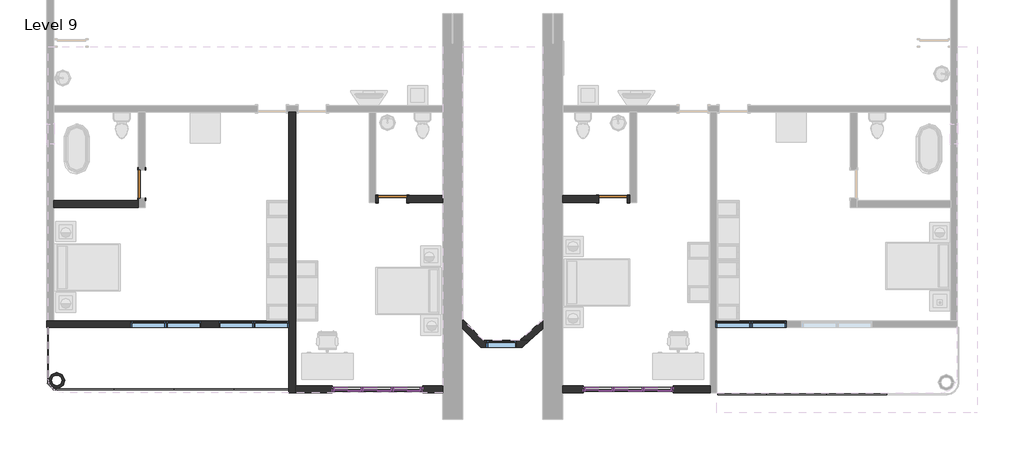
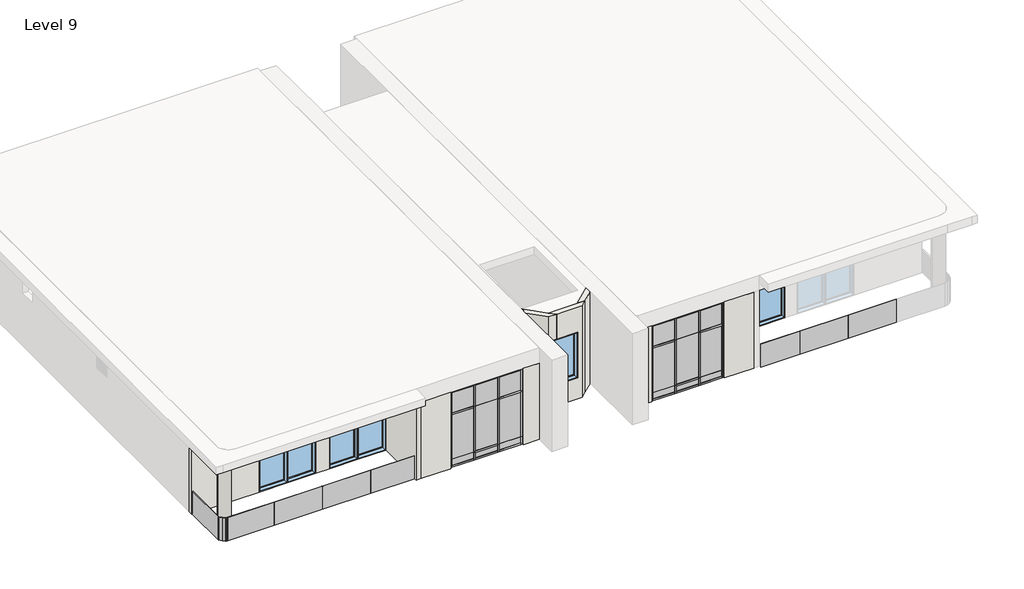
# One storey, part 1 of 3: 42 members, 30 plates, 14 walls, 7 windows, 3 doors.
"""IFC4 building model written with IfcOpenShell, lengths in millimetres."""

from ifc_helpers import new_model, si_unit, point, frame, frame_2d, origin, place, context, project, spatial, polyline, circle_curve, trimmed, segment, composite_curve, outline, extrude, faceted_brep, transform, mapped, element, save
from components import door_2703ae13, door_10fd3a06, member_c17f1be2, member_ad567e07, member_d2e7e466, member_7db1855a, member_75d1e245, member_d60e8053, member_3c3dc66a, member_2fae0574, member_410c6227, member_73c23c35, system_panel_glazed_38d54ecf, system_panel_glazed_fbb6c980, system_panel_glazed_4137532c, system_panel_glazed_6230de04, system_panel_glazed_a79f7f85, system_panel_glazed_9a5ea490, system_panel_glazed_95be5de7, system_panel_glazed_1e00a1c5, system_panel_glazed_ffe51582, system_panel_glazed_8f95e3f6, system_panel_glazed_836907cd, system_panel_glazed_688a65a2, system_panel_glazed_c1a1c740, system_panel_glazed_22bcd51f, window_9a779fa2, window_1a213a25

model = new_model("IFC4")

# Units and contexts
model_context = context("Model", 3, world=origin())
ifc_project = project(units=[si_unit("LENGTHUNIT", "METRE", prefix="MILLI")], contexts=[model_context])

# Site, building, storey
site = spatial("IfcSite", under=ifc_project)
building = spatial("IfcBuilding", under=site)
storey = spatial("IfcBuildingStorey", under=building, Name="Level 9", Elevation=29260.8)

# Doors
placement = place(None, origin())
door_shape = door_2703ae13(model_context)
element("IfcDoor", 1, ObjectType="Door-Single-Panel.0001 : 34\" x 80\"", at=placement, inside=storey, context=model_context, shape_type="MappedRepresentation", body=[
    mapped(door_shape, transform((-15765.9987704, -441.9241442, 29260.8), x_axis=(0.0, -1.0, 0.0), y_axis=(1.0, 0.0, 0.0), z_axis=(0.0, 0.0, 1.0))),
])
element("IfcDoor", 2, ObjectType="Door-Single-Panel.0001 : 34\" x 80\"", at=placement, inside=storey, context=model_context, shape_type="MappedRepresentation", body=[
    mapped(door_shape, transform((-8145.9987704, -899.1241442, 29260.8), x_axis=(-1.0, 0.0, 0.0), y_axis=(0.0, -1.0, 0.0), z_axis=(0.0, 0.0, 1.0))),
])
door_2_shape = door_10fd3a06(model_context)
element("IfcDoor", 3, ObjectType="Door-Single-Panel.0001 : 34\" x 80\"", at=placement, inside=storey, context=model_context, shape_type="MappedRepresentation", body=[
    mapped(door_2_shape, transform((-1440.3987704, -899.1241442, 29260.8), x_axis=(1.0, 0.0, 0.0), y_axis=(0.0, 1.0, 0.0), z_axis=(0.0, 0.0, 1.0))),
])

# Members
member_shape = member_c17f1be2(model_context)
element("IfcMember", 4, ObjectType="Rectangular Mullion : 2.5\" x 5\" rectangular", at=placement, inside=storey, context=model_context, shape_type="MappedRepresentation", body=[
    mapped(member_shape, transform((-9911.2987704, -6690.3241442, 32308.8), x_axis=(0.0, 0.0, 1.0), y_axis=(0.0, 1.0, 0.0), z_axis=(-1.0, 0.0, 0.0))),
])
element("IfcMember", 5, ObjectType="Rectangular Mullion : 2.5\" x 5\" rectangular", at=placement, inside=storey, context=model_context, shape_type="MappedRepresentation", body=[
    mapped(member_shape, transform((-8114.2487704, -6690.3241442, 32308.8), x_axis=(0.0, 0.0, 1.0), y_axis=(0.0, 1.0, 0.0), z_axis=(-1.0, 0.0, 0.0))),
])
element("IfcMember", 6, ObjectType="Rectangular Mullion : 2.5\" x 5\" rectangular", at=placement, inside=storey, context=model_context, shape_type="MappedRepresentation", body=[
    mapped(member_shape, transform((-2291.2987704, -6690.3241442, 32308.8), x_axis=(0.0, 0.0, 1.0), y_axis=(0.0, 1.0, 0.0), z_axis=(-1.0, 0.0, 0.0))),
])
element("IfcMember", 7, ObjectType="Rectangular Mullion : 2.5\" x 5\" rectangular", at=placement, inside=storey, context=model_context, shape_type="MappedRepresentation", body=[
    mapped(member_shape, transform((-494.2487704, -6690.3241442, 32308.8), x_axis=(0.0, 0.0, 1.0), y_axis=(0.0, 1.0, 0.0), z_axis=(-1.0, 0.0, 0.0))),
])
element("IfcMember", 8, ObjectType="Rectangular Mullion : 2.5\" x 5\" rectangular", at=placement, inside=storey, context=model_context, shape_type="MappedRepresentation", body=[
    mapped(member_shape, transform((-7295.0987704, -6690.3241442, 29260.8), x_axis=(0.0, 0.0, -1.0), y_axis=(0.0, 1.0, 0.0), z_axis=(1.0, 0.0, 0.0))),
])
element("IfcMember", 9, ObjectType="Rectangular Mullion : 2.5\" x 5\" rectangular", at=placement, inside=storey, context=model_context, shape_type="MappedRepresentation", body=[
    mapped(member_shape, transform((-9092.1487704, -6690.3241442, 29260.8), x_axis=(0.0, 0.0, -1.0), y_axis=(0.0, 1.0, 0.0), z_axis=(1.0, 0.0, 0.0))),
])
element("IfcMember", 10, ObjectType="Rectangular Mullion : 2.5\" x 5\" rectangular", at=placement, inside=storey, context=model_context, shape_type="MappedRepresentation", body=[
    mapped(member_shape, transform((324.9012296, -6690.3241442, 29260.8), x_axis=(0.0, 0.0, -1.0), y_axis=(0.0, 1.0, 0.0), z_axis=(1.0, 0.0, 0.0))),
])
element("IfcMember", 11, ObjectType="Rectangular Mullion : 2.5\" x 5\" rectangular", at=placement, inside=storey, context=model_context, shape_type="MappedRepresentation", body=[
    mapped(member_shape, transform((-1472.1487704, -6690.3241442, 29260.8), x_axis=(0.0, 0.0, -1.0), y_axis=(0.0, 1.0, 0.0), z_axis=(1.0, 0.0, 0.0))),
])
member_2_shape = member_ad567e07(model_context)
element("IfcMember", 12, ObjectType="Rectangular Mullion : 2.5\" x 5\" rectangular", at=placement, inside=storey, context=model_context, shape_type="MappedRepresentation", body=[
    mapped(member_2_shape, transform((-8114.2487704, -6690.3241442, 31394.4), x_axis=(0.0, 0.0, 1.0), y_axis=(0.0, 1.0, 0.0), z_axis=(-1.0, 0.0, 0.0))),
])
element("IfcMember", 13, ObjectType="Rectangular Mullion : 2.5\" x 5\" rectangular", at=placement, inside=storey, context=model_context, shape_type="MappedRepresentation", body=[
    mapped(member_2_shape, transform((-9911.2987704, -6690.3241442, 31394.4), x_axis=(0.0, 0.0, 1.0), y_axis=(0.0, 1.0, 0.0), z_axis=(-1.0, 0.0, 0.0))),
])
element("IfcMember", 14, ObjectType="Rectangular Mullion : 2.5\" x 5\" rectangular", at=placement, inside=storey, context=model_context, shape_type="MappedRepresentation", body=[
    mapped(member_2_shape, transform((-494.2487704, -6690.3241442, 31394.4), x_axis=(0.0, 0.0, 1.0), y_axis=(0.0, 1.0, 0.0), z_axis=(-1.0, 0.0, 0.0))),
])
element("IfcMember", 15, ObjectType="Rectangular Mullion : 2.5\" x 5\" rectangular", at=placement, inside=storey, context=model_context, shape_type="MappedRepresentation", body=[
    mapped(member_2_shape, transform((-2291.2987704, -6690.3241442, 31394.4), x_axis=(0.0, 0.0, 1.0), y_axis=(0.0, 1.0, 0.0), z_axis=(-1.0, 0.0, 0.0))),
])
member_3_shape = member_d2e7e466(model_context)
element("IfcMember", 16, ObjectType="Rectangular Mullion : 2.5\" x 5\" rectangular", at=placement, inside=storey, context=model_context, shape_type="MappedRepresentation", body=[
    mapped(member_3_shape, transform((-8177.7487704, -6690.3241442, 29260.8), x_axis=(0.0, 0.0, -1.0), y_axis=(0.0, 1.0, 0.0), z_axis=(1.0, 0.0, 0.0))),
])
element("IfcMember", 17, ObjectType="Rectangular Mullion : 2.5\" x 5\" rectangular", at=placement, inside=storey, context=model_context, shape_type="MappedRepresentation", body=[
    mapped(member_3_shape, transform((-557.7487704, -6690.3241442, 29260.8), x_axis=(0.0, 0.0, -1.0), y_axis=(0.0, 1.0, 0.0), z_axis=(1.0, 0.0, 0.0))),
])
member_4_shape = member_7db1855a(model_context)
element("IfcMember", 18, ObjectType="Rectangular Mullion : 2.5\" x 5\" rectangular", at=placement, inside=storey, context=model_context, shape_type="MappedRepresentation", body=[
    mapped(member_4_shape, transform((-9028.6487704, -6690.3241442, 29565.6), x_axis=(0.0, 0.0, 1.0), y_axis=(0.0, 1.0, 0.0), z_axis=(-1.0, 0.0, 0.0))),
])
element("IfcMember", 19, ObjectType="Rectangular Mullion : 2.5\" x 5\" rectangular", at=placement, inside=storey, context=model_context, shape_type="MappedRepresentation", body=[
    mapped(member_4_shape, transform((-1408.6487704, -6690.3241442, 29565.6), x_axis=(0.0, 0.0, 1.0), y_axis=(0.0, 1.0, 0.0), z_axis=(-1.0, 0.0, 0.0))),
])
element("IfcMember", 20, ObjectType="Rectangular Mullion : 2.5\" x 5\" rectangular", at=placement, inside=storey, context=model_context, shape_type="MappedRepresentation", body=[
    mapped(member_3_shape, transform((-9028.6487704, -6690.3241442, 32308.8), x_axis=(0.0, 0.0, 1.0), y_axis=(0.0, 1.0, 0.0), z_axis=(-1.0, 0.0, 0.0))),
])
element("IfcMember", 21, ObjectType="Rectangular Mullion : 2.5\" x 5\" rectangular", at=placement, inside=storey, context=model_context, shape_type="MappedRepresentation", body=[
    mapped(member_3_shape, transform((-1408.6487704, -6690.3241442, 32308.8), x_axis=(0.0, 0.0, 1.0), y_axis=(0.0, 1.0, 0.0), z_axis=(-1.0, 0.0, 0.0))),
])
member_5_shape = member_75d1e245(model_context)
element("IfcMember", 22, ObjectType="Rectangular Mullion : 2.5\" x 5\" rectangular", at=placement, inside=storey, context=model_context, shape_type="MappedRepresentation", body=[
    mapped(member_5_shape, transform((-8145.9987704, -6690.3241442, 29260.8), x_axis=(-1.0, 0.0, 0.0), y_axis=(0.0, 1.0, 0.0), z_axis=(0.0, 0.0, -1.0))),
])
element("IfcMember", 23, ObjectType="Rectangular Mullion : 2.5\" x 5\" rectangular", at=placement, inside=storey, context=model_context, shape_type="MappedRepresentation", body=[
    mapped(member_5_shape, transform((-9060.3987704, -6690.3241442, 29260.8), x_axis=(-1.0, 0.0, 0.0), y_axis=(0.0, 1.0, 0.0), z_axis=(0.0, 0.0, -1.0))),
])
element("IfcMember", 24, ObjectType="Rectangular Mullion : 2.5\" x 5\" rectangular", at=placement, inside=storey, context=model_context, shape_type="MappedRepresentation", body=[
    mapped(member_5_shape, transform((-525.9987704, -6690.3241442, 29260.8), x_axis=(-1.0, 0.0, 0.0), y_axis=(0.0, 1.0, 0.0), z_axis=(0.0, 0.0, -1.0))),
])
element("IfcMember", 25, ObjectType="Rectangular Mullion : 2.5\" x 5\" rectangular", at=placement, inside=storey, context=model_context, shape_type="MappedRepresentation", body=[
    mapped(member_5_shape, transform((-1440.3987704, -6690.3241442, 29260.8), x_axis=(-1.0, 0.0, 0.0), y_axis=(0.0, 1.0, 0.0), z_axis=(0.0, 0.0, -1.0))),
])
member_6_shape = member_d60e8053(model_context)
element("IfcMember", 26, ObjectType="Rectangular Mullion : 2.5\" x 5\" rectangular", at=placement, inside=storey, context=model_context, shape_type="MappedRepresentation", body=[
    mapped(member_6_shape, transform((-8145.9987704, -6690.3241442, 29565.6), x_axis=(-1.0, 0.0, 0.0), y_axis=(0.0, 1.0, 0.0), z_axis=(0.0, 0.0, -1.0))),
])
element("IfcMember", 27, ObjectType="Rectangular Mullion : 2.5\" x 5\" rectangular", at=placement, inside=storey, context=model_context, shape_type="MappedRepresentation", body=[
    mapped(member_6_shape, transform((-9060.3987704, -6690.3241442, 29565.6), x_axis=(-1.0, 0.0, 0.0), y_axis=(0.0, 1.0, 0.0), z_axis=(0.0, 0.0, -1.0))),
])
element("IfcMember", 28, ObjectType="Rectangular Mullion : 2.5\" x 5\" rectangular", at=placement, inside=storey, context=model_context, shape_type="MappedRepresentation", body=[
    mapped(member_6_shape, transform((-525.9987704, -6690.3241442, 29565.6), x_axis=(-1.0, 0.0, 0.0), y_axis=(0.0, 1.0, 0.0), z_axis=(0.0, 0.0, -1.0))),
])
element("IfcMember", 29, ObjectType="Rectangular Mullion : 2.5\" x 5\" rectangular", at=placement, inside=storey, context=model_context, shape_type="MappedRepresentation", body=[
    mapped(member_6_shape, transform((-1440.3987704, -6690.3241442, 29565.6), x_axis=(-1.0, 0.0, 0.0), y_axis=(0.0, 1.0, 0.0), z_axis=(0.0, 0.0, -1.0))),
])
member_7_shape = member_3c3dc66a(model_context)
element("IfcMember", 30, ObjectType="Rectangular Mullion : 2.5\" x 5\" rectangular", at=placement, inside=storey, context=model_context, shape_type="MappedRepresentation", body=[
    mapped(member_7_shape, transform((-9974.7987704, -6690.3241442, 29260.8), x_axis=(-1.0, 0.0, 0.0), y_axis=(0.0, 1.0, 0.0), z_axis=(0.0, 0.0, -1.0))),
])
element("IfcMember", 31, ObjectType="Rectangular Mullion : 2.5\" x 5\" rectangular", at=placement, inside=storey, context=model_context, shape_type="MappedRepresentation", body=[
    mapped(member_7_shape, transform((-2354.7987704, -6690.3241442, 29260.8), x_axis=(-1.0, 0.0, 0.0), y_axis=(0.0, 1.0, 0.0), z_axis=(0.0, 0.0, -1.0))),
])
member_8_shape = member_2fae0574(model_context)
element("IfcMember", 32, ObjectType="Rectangular Mullion : 2.5\" x 5\" rectangular", at=placement, inside=storey, context=model_context, shape_type="MappedRepresentation", body=[
    mapped(member_8_shape, transform((-9974.7987704, -6690.3241442, 29565.6), x_axis=(-1.0, 0.0, 0.0), y_axis=(0.0, 1.0, 0.0), z_axis=(0.0, 0.0, -1.0))),
])
element("IfcMember", 33, ObjectType="Rectangular Mullion : 2.5\" x 5\" rectangular", at=placement, inside=storey, context=model_context, shape_type="MappedRepresentation", body=[
    mapped(member_8_shape, transform((-2354.7987704, -6690.3241442, 29565.6), x_axis=(-1.0, 0.0, 0.0), y_axis=(0.0, 1.0, 0.0), z_axis=(0.0, 0.0, -1.0))),
])
element("IfcMember", 34, ObjectType="Rectangular Mullion : 2.5\" x 5\" rectangular", at=placement, inside=storey, context=model_context, shape_type="MappedRepresentation", body=[
    mapped(member_8_shape, transform((-7231.5987704, -6690.3241442, 31394.4), x_axis=(1.0, 0.0, 0.0), y_axis=(0.0, 1.0, 0.0), z_axis=(0.0, 0.0, 1.0))),
])
element("IfcMember", 35, ObjectType="Rectangular Mullion : 2.5\" x 5\" rectangular", at=placement, inside=storey, context=model_context, shape_type="MappedRepresentation", body=[
    mapped(member_8_shape, transform((388.4012296, -6690.3241442, 31394.4), x_axis=(1.0, 0.0, 0.0), y_axis=(0.0, 1.0, 0.0), z_axis=(0.0, 0.0, 1.0))),
])
element("IfcMember", 36, ObjectType="Rectangular Mullion : 2.5\" x 5\" rectangular", at=placement, inside=storey, context=model_context, shape_type="MappedRepresentation", body=[
    mapped(member_7_shape, transform((-7231.5987704, -6690.3241442, 29565.6), x_axis=(1.0, 0.0, 0.0), y_axis=(0.0, 1.0, 0.0), z_axis=(0.0, 0.0, 1.0))),
])
element("IfcMember", 37, ObjectType="Rectangular Mullion : 2.5\" x 5\" rectangular", at=placement, inside=storey, context=model_context, shape_type="MappedRepresentation", body=[
    mapped(member_7_shape, transform((388.4012296, -6690.3241442, 29565.6), x_axis=(1.0, 0.0, 0.0), y_axis=(0.0, 1.0, 0.0), z_axis=(0.0, 0.0, 1.0))),
])
member_9_shape = member_410c6227(model_context)
element("IfcMember", 38, ObjectType="Rectangular Mullion : 2.5\" x 5\" rectangular", at=placement, inside=storey, context=model_context, shape_type="MappedRepresentation", body=[
    mapped(member_9_shape, transform((-8145.9987704, -6690.3241442, 31394.4), x_axis=(-1.0, 0.0, 0.0), y_axis=(0.0, 1.0, 0.0), z_axis=(0.0, 0.0, -1.0))),
])
element("IfcMember", 39, ObjectType="Rectangular Mullion : 2.5\" x 5\" rectangular", at=placement, inside=storey, context=model_context, shape_type="MappedRepresentation", body=[
    mapped(member_9_shape, transform((-9060.3987704, -6690.3241442, 31394.4), x_axis=(-1.0, 0.0, 0.0), y_axis=(0.0, 1.0, 0.0), z_axis=(0.0, 0.0, -1.0))),
])
element("IfcMember", 40, ObjectType="Rectangular Mullion : 2.5\" x 5\" rectangular", at=placement, inside=storey, context=model_context, shape_type="MappedRepresentation", body=[
    mapped(member_9_shape, transform((-525.9987704, -6690.3241442, 31394.4), x_axis=(-1.0, 0.0, 0.0), y_axis=(0.0, 1.0, 0.0), z_axis=(0.0, 0.0, -1.0))),
])
element("IfcMember", 41, ObjectType="Rectangular Mullion : 2.5\" x 5\" rectangular", at=placement, inside=storey, context=model_context, shape_type="MappedRepresentation", body=[
    mapped(member_9_shape, transform((-1440.3987704, -6690.3241442, 31394.4), x_axis=(-1.0, 0.0, 0.0), y_axis=(0.0, 1.0, 0.0), z_axis=(0.0, 0.0, -1.0))),
])
member_10_shape = member_73c23c35(model_context)
element("IfcMember", 42, ObjectType="Rectangular Mullion : 2.5\" x 5\" rectangular", at=placement, inside=storey, context=model_context, shape_type="MappedRepresentation", body=[
    mapped(member_10_shape, transform((-7231.5987704, -6690.3241442, 32308.8), x_axis=(1.0, 0.0, 0.0), y_axis=(0.0, 1.0, 0.0), z_axis=(0.0, 0.0, 1.0))),
])
element("IfcMember", 43, ObjectType="Rectangular Mullion : 2.5\" x 5\" rectangular", at=placement, inside=storey, context=model_context, shape_type="MappedRepresentation", body=[
    mapped(member_10_shape, transform((388.4012296, -6690.3241442, 32308.8), x_axis=(1.0, 0.0, 0.0), y_axis=(0.0, 1.0, 0.0), z_axis=(0.0, 0.0, 1.0))),
])
element("IfcMember", 44, ObjectType="Rectangular Mullion : 2.5\" x 5\" rectangular", at=placement, inside=storey, context=model_context, shape_type="MappedRepresentation", body=[
    mapped(member_10_shape, transform((-9974.7987704, -6690.3241442, 31394.4), x_axis=(-1.0, 0.0, 0.0), y_axis=(0.0, 1.0, 0.0), z_axis=(0.0, 0.0, -1.0))),
])
element("IfcMember", 45, ObjectType="Rectangular Mullion : 2.5\" x 5\" rectangular", at=placement, inside=storey, context=model_context, shape_type="MappedRepresentation", body=[
    mapped(member_10_shape, transform((-2354.7987704, -6690.3241442, 31394.4), x_axis=(-1.0, 0.0, 0.0), y_axis=(0.0, 1.0, 0.0), z_axis=(0.0, 0.0, -1.0))),
])

# Plates
system_panel_glazed_shape = system_panel_glazed_38d54ecf(model_context)
element("IfcPlate", 46, ObjectType="System Panel : Glazed", at=placement, inside=storey, context=model_context, shape_type="MappedRepresentation", body=[
    mapped(system_panel_glazed_shape, transform((-8603.1987704, -6690.3241442, 29597.35), x_axis=(-1.0, 0.0, 0.0), y_axis=(0.0, -1.0, 0.0), z_axis=(0.0, 0.0, 1.0))),
])
element("IfcPlate", 47, ObjectType="System Panel : Glazed", at=placement, inside=storey, context=model_context, shape_type="MappedRepresentation", body=[
    mapped(system_panel_glazed_shape, transform((-983.1987704, -6690.3241442, 29597.35), x_axis=(-1.0, 0.0, 0.0), y_axis=(0.0, -1.0, 0.0), z_axis=(0.0, 0.0, 1.0))),
])
system_panel_glazed_2_shape = system_panel_glazed_fbb6c980(model_context)
element("IfcPlate", 48, ObjectType="System Panel : Glazed", at=placement, inside=storey, context=model_context, shape_type="MappedRepresentation", body=[
    mapped(system_panel_glazed_2_shape, transform((-8603.1987704, -6690.3241442, 29324.3), x_axis=(-1.0, 0.0, 0.0), y_axis=(0.0, -1.0, 0.0), z_axis=(0.0, 0.0, 1.0))),
])
element("IfcPlate", 49, ObjectType="System Panel : Glazed", at=placement, inside=storey, context=model_context, shape_type="MappedRepresentation", body=[
    mapped(system_panel_glazed_2_shape, transform((-983.1987704, -6690.3241442, 29324.3), x_axis=(-1.0, 0.0, 0.0), y_axis=(0.0, -1.0, 0.0), z_axis=(0.0, 0.0, 1.0))),
])
system_panel_glazed_3_shape = system_panel_glazed_4137532c(model_context)
element("IfcPlate", 50, ObjectType="System Panel : Glazed", at=placement, inside=storey, context=model_context, shape_type="MappedRepresentation", body=[
    mapped(system_panel_glazed_3_shape, transform((-7704.6737704, -6690.3241442, 29324.3), x_axis=(-1.0, 0.0, 0.0), y_axis=(0.0, -1.0, 0.0), z_axis=(0.0, 0.0, 1.0))),
])
element("IfcPlate", 51, ObjectType="System Panel : Glazed", at=placement, inside=storey, context=model_context, shape_type="MappedRepresentation", body=[
    mapped(system_panel_glazed_3_shape, transform((-9501.7237704, -6690.3241442, 29324.3), x_axis=(-1.0, 0.0, 0.0), y_axis=(0.0, -1.0, 0.0), z_axis=(0.0, 0.0, 1.0))),
])
element("IfcPlate", 52, ObjectType="System Panel : Glazed", at=placement, inside=storey, context=model_context, shape_type="MappedRepresentation", body=[
    mapped(system_panel_glazed_3_shape, transform((-84.6737704, -6690.3241442, 29324.3), x_axis=(-1.0, 0.0, 0.0), y_axis=(0.0, -1.0, 0.0), z_axis=(0.0, 0.0, 1.0))),
])
element("IfcPlate", 53, ObjectType="System Panel : Glazed", at=placement, inside=storey, context=model_context, shape_type="MappedRepresentation", body=[
    mapped(system_panel_glazed_3_shape, transform((-1881.7237704, -6690.3241442, 29324.3), x_axis=(-1.0, 0.0, 0.0), y_axis=(0.0, -1.0, 0.0), z_axis=(0.0, 0.0, 1.0))),
])
system_panel_glazed_4_shape = system_panel_glazed_6230de04(model_context)
element("IfcPlate", 54, ObjectType="System Panel : Glazed", at=placement, inside=storey, context=model_context, shape_type="MappedRepresentation", body=[
    mapped(system_panel_glazed_4_shape, transform((-7704.6737704, -6690.3241442, 29565.6), x_axis=(-1.0, 0.0, 0.0), y_axis=(0.0, -1.0, 0.0), z_axis=(0.0, 0.0, 1.0))),
])
element("IfcPlate", 55, ObjectType="System Panel : Glazed", at=placement, inside=storey, context=model_context, shape_type="MappedRepresentation", body=[
    mapped(system_panel_glazed_4_shape, transform((-9501.7237704, -6690.3241442, 29565.6), x_axis=(-1.0, 0.0, 0.0), y_axis=(0.0, -1.0, 0.0), z_axis=(0.0, 0.0, 1.0))),
])
element("IfcPlate", 56, ObjectType="System Panel : Glazed", at=placement, inside=storey, context=model_context, shape_type="MappedRepresentation", body=[
    mapped(system_panel_glazed_4_shape, transform((-84.6737704, -6690.3241442, 29565.6), x_axis=(-1.0, 0.0, 0.0), y_axis=(0.0, -1.0, 0.0), z_axis=(0.0, 0.0, 1.0))),
])
element("IfcPlate", 57, ObjectType="System Panel : Glazed", at=placement, inside=storey, context=model_context, shape_type="MappedRepresentation", body=[
    mapped(system_panel_glazed_4_shape, transform((-1881.7237704, -6690.3241442, 29565.6), x_axis=(-1.0, 0.0, 0.0), y_axis=(0.0, -1.0, 0.0), z_axis=(0.0, 0.0, 1.0))),
])
system_panel_glazed_5_shape = system_panel_glazed_a79f7f85(model_context)
element("IfcPlate", 58, ObjectType="System Panel : Glazed", at=placement, inside=storey, context=model_context, shape_type="MappedRepresentation", body=[
    mapped(system_panel_glazed_5_shape, transform((-7704.6737704, -6690.3241442, 31426.15), x_axis=(-1.0, 0.0, 0.0), y_axis=(0.0, -1.0, 0.0), z_axis=(0.0, 0.0, 1.0))),
])
element("IfcPlate", 59, ObjectType="System Panel : Glazed", at=placement, inside=storey, context=model_context, shape_type="MappedRepresentation", body=[
    mapped(system_panel_glazed_5_shape, transform((-9501.7237704, -6690.3241442, 31426.15), x_axis=(-1.0, 0.0, 0.0), y_axis=(0.0, -1.0, 0.0), z_axis=(0.0, 0.0, 1.0))),
])
element("IfcPlate", 60, ObjectType="System Panel : Glazed", at=placement, inside=storey, context=model_context, shape_type="MappedRepresentation", body=[
    mapped(system_panel_glazed_5_shape, transform((-84.6737704, -6690.3241442, 31426.15), x_axis=(-1.0, 0.0, 0.0), y_axis=(0.0, -1.0, 0.0), z_axis=(0.0, 0.0, 1.0))),
])
element("IfcPlate", 61, ObjectType="System Panel : Glazed", at=placement, inside=storey, context=model_context, shape_type="MappedRepresentation", body=[
    mapped(system_panel_glazed_5_shape, transform((-1881.7237704, -6690.3241442, 31426.15), x_axis=(-1.0, 0.0, 0.0), y_axis=(0.0, -1.0, 0.0), z_axis=(0.0, 0.0, 1.0))),
])
system_panel_glazed_6_shape = system_panel_glazed_9a5ea490(model_context)
element("IfcPlate", 62, ObjectType="System Panel : Glazed", at=placement, inside=storey, context=model_context, shape_type="MappedRepresentation", body=[
    mapped(system_panel_glazed_6_shape, transform((-8603.1987704, -6690.3241442, 31394.4), x_axis=(-1.0, 0.0, 0.0), y_axis=(0.0, -1.0, 0.0), z_axis=(0.0, 0.0, 1.0))),
])
element("IfcPlate", 63, ObjectType="System Panel : Glazed", at=placement, inside=storey, context=model_context, shape_type="MappedRepresentation", body=[
    mapped(system_panel_glazed_6_shape, transform((-983.1987704, -6690.3241442, 31394.4), x_axis=(-1.0, 0.0, 0.0), y_axis=(0.0, -1.0, 0.0), z_axis=(0.0, 0.0, 1.0))),
])
system_panel_glazed_7_shape = system_panel_glazed_95be5de7(model_context)
element("IfcPlate", 64, ObjectType="System Panel : Glazed", at=placement, inside=storey, context=model_context, shape_type="MappedRepresentation", body=[
    mapped(system_panel_glazed_7_shape, transform((-15707.2305745, -6723.6923401, 29260.8), x_axis=(1.0, 0.0, 0.0), y_axis=(0.0, 1.0, 0.0), z_axis=(0.0, 0.0, 1.0))),
])
element("IfcPlate", 65, ObjectType="System Panel : Glazed", at=placement, inside=storey, context=model_context, shape_type="MappedRepresentation", body=[
    mapped(system_panel_glazed_7_shape, transform((-13878.4305745, -6723.6923401, 29260.8), x_axis=(1.0, 0.0, 0.0), y_axis=(0.0, 1.0, 0.0), z_axis=(0.0, 0.0, 1.0))),
])
element("IfcPlate", 66, ObjectType="System Panel : Glazed", at=placement, inside=storey, context=model_context, shape_type="MappedRepresentation", body=[
    mapped(system_panel_glazed_7_shape, transform((5957.9120092, -6810.4133646, 29260.8), x_axis=(-1.0, 0.0, 0.0), y_axis=(0.0, -1.0, 0.0), z_axis=(0.0, 0.0, 1.0))),
])
element("IfcPlate", 67, ObjectType="System Panel : Glazed", at=placement, inside=storey, context=model_context, shape_type="MappedRepresentation", body=[
    mapped(system_panel_glazed_7_shape, transform((4129.1120092, -6810.4133646, 29260.8), x_axis=(-1.0, 0.0, 0.0), y_axis=(0.0, -1.0, 0.0), z_axis=(0.0, 0.0, 1.0))),
])
system_panel_glazed_8_shape = system_panel_glazed_1e00a1c5(model_context)
element("IfcPlate", 68, ObjectType="System Panel : Glazed", at=placement, inside=storey, context=model_context, shape_type="MappedRepresentation", body=[
    mapped(system_panel_glazed_8_shape, transform((2478.1120092, -6810.4133646, 29260.8), x_axis=(-1.0, 0.0, 0.0), y_axis=(0.0, -1.0, 0.0), z_axis=(0.0, 0.0, 1.0))),
])
system_panel_glazed_9_shape = system_panel_glazed_ffe51582(model_context)
element("IfcPlate", 69, ObjectType="System Panel : Glazed", at=placement, inside=storey, context=model_context, shape_type="MappedRepresentation", body=[
    mapped(system_panel_glazed_9_shape, transform((-18451.9713429, -6722.1515718, 29260.8), x_axis=(0.7071067811865462, -0.7071067811865488, 0.0), y_axis=(0.7071067811865488, 0.7071067811865462, 0.0), z_axis=(0.0, 0.0, 1.0))),
])
system_panel_glazed_10_shape = system_panel_glazed_8f95e3f6(model_context)
element("IfcPlate", 70, ObjectType="System Panel : Glazed", at=placement, inside=storey, context=model_context, shape_type="MappedRepresentation", body=[
    mapped(system_panel_glazed_10_shape, transform((-18648.8987704, -5667.9741442, 29260.8), x_axis=(0.0, -1.0, 0.0), y_axis=(1.0, 0.0, 0.0), z_axis=(0.0, 0.0, 1.0))),
])
system_panel_glazed_11_shape = system_panel_glazed_836907cd(model_context)
element("IfcPlate", 71, ObjectType="System Panel : Glazed", at=placement, inside=storey, context=model_context, shape_type="MappedRepresentation", body=[
    mapped(system_panel_glazed_11_shape, transform((-18418.6805745, -6723.6923401, 29260.8), x_axis=(1.0, 0.0, 0.0), y_axis=(0.0, 1.0, 0.0), z_axis=(0.0, 0.0, 1.0))),
])
system_panel_glazed_12_shape = system_panel_glazed_688a65a2(model_context)
element("IfcPlate", 72, ObjectType="System Panel : Glazed", at=placement, inside=storey, context=model_context, shape_type="MappedRepresentation", body=[
    mapped(system_panel_glazed_12_shape, transform((-12129.8146725, -6723.6923401, 29260.8), x_axis=(1.0, 0.0, 0.0), y_axis=(0.0, 1.0, 0.0), z_axis=(0.0, 0.0, 1.0))),
])
system_panel_glazed_13_shape = system_panel_glazed_c1a1c740(model_context)
element("IfcPlate", 73, ObjectType="System Panel : Glazed", at=placement, inside=storey, context=model_context, shape_type="MappedRepresentation", body=[
    mapped(system_panel_glazed_13_shape, transform((-17504.2805745, -6723.6923401, 29260.8), x_axis=(1.0, 0.0, 0.0), y_axis=(0.0, 1.0, 0.0), z_axis=(0.0, 0.0, 1.0))),
])
system_panel_glazed_14_shape = system_panel_glazed_22bcd51f(model_context)
element("IfcPlate", 74, ObjectType="System Panel : Glazed", at=placement, inside=storey, context=model_context, shape_type="MappedRepresentation", body=[
    mapped(system_panel_glazed_14_shape, transform((-18600.0521056, -6574.070809, 29260.8), x_axis=(0.7071067811865462, -0.7071067811865488, 0.0), y_axis=(0.7071067811865488, 0.7071067811865462, 0.0), z_axis=(0.0, 0.0, 1.0))),
])
element("IfcPlate", 75, ObjectType="System Panel : Glazed", at=placement, inside=storey, context=model_context, shape_type="MappedRepresentation", body=[
    mapped(system_panel_glazed_14_shape, transform((-18502.3587761, -6671.7641386, 29260.8), x_axis=(0.7071067811865462, -0.7071067811865488, 0.0), y_axis=(0.7071067811865488, 0.7071067811865462, 0.0), z_axis=(0.0, 0.0, 1.0))),
])

# Walls
element("IfcWall", 76, ObjectType="Generic - 3\" green 2", at=placement, inside=storey, context=model_context, shape_type="SweptSolid", body=[
    extrude(outline(composite_curve([segment(polyline([(-18518.7237704, -6418.8616442), (-18594.9237704, -6418.8616442)]), True, "CONTINUOUS"), segment(trimmed(circle_curve(frame_2d((-18353.6237704, -6418.8616442)), 241.3), [point((-18594.9237704, -6418.8616442))], [point((-18112.3237704, -6418.8616442))], False, "CARTESIAN"), True, "CONTINUOUS"), segment(polyline([(-18112.3237704, -6418.8616442), (-18188.5237704, -6418.8616442)]), True, "CONTINUOUS"), segment(trimmed(circle_curve(frame_2d((-18353.6237704, -6418.8616442)), 165.1), [point((-18188.5237704, -6418.8616442))], [point((-18518.7237704, -6418.8616442))], True, "CARTESIAN"), True, "CONTINUOUS")], self_intersect=False)), frame((0.0, 0.0, 29260.8), z_axis=(0.0, 0.0, 1.0), x_axis=(1.0, 0.0, 0.0)), (0.0, 0.0, 1.0), 3048.0),
])
element("IfcWall", 77, ObjectType="Generic - 3\" green 2", at=placement, inside=storey, context=model_context, shape_type="SweptSolid", body=[
    extrude(outline(composite_curve([segment(polyline([(-18188.5237704, -6418.8616442), (-18112.3237704, -6418.8616442)]), True, "CONTINUOUS"), segment(trimmed(circle_curve(frame_2d((-18353.6237704, -6418.8616442)), 241.3), [point((-18112.3237704, -6418.8616442))], [point((-18594.9237704, -6418.8616442))], False, "CARTESIAN"), True, "CONTINUOUS"), segment(polyline([(-18594.9237704, -6418.8616442), (-18518.7237704, -6418.8616442)]), True, "CONTINUOUS"), segment(trimmed(circle_curve(frame_2d((-18353.6237704, -6418.8616442)), 165.1), [point((-18518.7237704, -6418.8616442))], [point((-18188.5237704, -6418.8616442))], True, "CARTESIAN"), True, "CONTINUOUS")], self_intersect=False)), frame((0.0, 0.0, 29260.8), z_axis=(0.0, 0.0, 1.0), x_axis=(1.0, 0.0, 0.0)), (0.0, 0.0, 1.0), 3048.0),
])
element("IfcWall", 78, ObjectType="Generic - 8\" cream", at=placement, inside=storey, context=model_context, shape_type="Brep", body=[
    faceted_brep([(-11295.5987704, 1742.4758558, 29260.8), (-11295.5987704, -6791.9241442, 29260.8), (-11295.5987704, -6791.9241442, 32308.8), (-11295.5987704, -4810.7241442, 32308.8), (-11295.5987704, -4607.5241442, 32308.8), (-11295.5987704, 1742.4758558, 32308.8), (-11092.3987704, 1742.4758558, 29260.8), (-11092.3987704, 1742.4758558, 32308.8), (-11092.3987704, -6588.7241442, 32308.8), (-11092.3987704, -6791.9241442, 32308.8), (-11092.3987704, -6791.9241442, 29260.8), (-11092.3987704, -6588.7241442, 29260.8)], [[[0, 1, 2, 3, 4, 5]], [[6, 7, 8, 9, 10, 11]], [[1, 0, 6, 11, 10]], [[5, 4, 3, 2, 9, 8, 7]], [[0, 5, 7, 6]], [[2, 1, 10, 9]]]),
])
element("IfcWall", 79, ObjectType="Generic - 8\" cream", at=placement, inside=storey, context=model_context, shape_type="SweptSolid", body=[
    extrude(outline(polyline([(-18445.6987704, -949.9241442), (-15867.5987704, -949.9241442), (-15867.5987704, -1153.1241442), (-18445.6987704, -1153.1241442), (-18445.6987704, -949.9241442)])), frame((0.0, 0.0, 29260.8), z_axis=(0.0, 0.0, 1.0), x_axis=(1.0, 0.0, 0.0)), (0.0, 0.0, 1.0), 3048.0),
])
element("IfcWall", 80, ObjectType="Generic - 8\" cream", at=placement, inside=storey, context=model_context, shape_type="SweptSolid", body=[
    extrude(outline(polyline([(32308.8, -6621.9987704), (32308.8, -8653.9987704), (29260.8, -8653.9987704), (29260.8, -8577.7987704), (31292.8, -8577.7987704), (31292.8, -7714.1987704), (29260.8, -7714.1987704), (29260.8, -6621.9987704), (32308.8, -6621.9987704)])), frame((0.0, -1000.7241442, 0.0), z_axis=(0.0, 1.0, 0.0), x_axis=(0.0, 0.0, 1.0)), (0.0, 0.0, 1.0), 203.2),
])
element("IfcWall", 81, ObjectType="Generic - 8\" cream", at=placement, inside=storey, context=model_context, shape_type="Brep", body=[
    faceted_brep([(-18648.8987704, -4607.5241442, 32308.8), (-18445.6987704, -4607.5241442, 32308.8), (-11295.5987704, -4607.5241442, 32308.8), (-11295.5987704, -4607.5241442, 32004.0), (-13429.1987704, -4607.5241442, 32004.0), (-13429.1987704, -4607.5241442, 29260.8), (-13962.5987704, -4607.5241442, 29260.8), (-13962.5987704, -4607.5241442, 32004.0), (-16096.1987704, -4607.5241442, 32004.0), (-16096.1987704, -4607.5241442, 29260.8), (-18445.6987704, -4607.5241442, 29260.8), (-18648.8987704, -4607.5241442, 29260.8), (-11295.5987704, -4810.7241442, 32308.8), (-18648.8987704, -4810.7241442, 32308.8), (-18648.8987704, -4810.7241442, 29260.8), (-16096.1987704, -4810.7241442, 29260.8), (-16096.1987704, -4810.7241442, 32004.0), (-13962.5987704, -4810.7241442, 32004.0), (-13962.5987704, -4810.7241442, 29260.8), (-13429.1987704, -4810.7241442, 29260.8), (-13429.1987704, -4810.7241442, 32004.0), (-11295.5987704, -4810.7241442, 32004.0)], [[[0, 1, 2, 3, 4, 5, 6, 7, 8, 9, 10, 11]], [[12, 13, 14, 15, 16, 17, 18, 19, 20, 21]], [[14, 11, 10, 9, 15]], [[5, 19, 18, 6]], [[2, 1, 0, 13, 12]], [[2, 12, 21, 3]], [[0, 11, 14, 13]], [[3, 21, 20, 4]], [[4, 20, 19, 5]], [[17, 7, 6, 18]], [[7, 17, 16, 8]], [[8, 16, 15, 9]]]),
])
element("IfcWall", 82, ObjectType="Generic - 8\" cream", at=placement, inside=storey, context=model_context, shape_type="SweptSolid", body=[
    extrude(outline(polyline([(32308.8, -932.3987704), (32308.8, -2964.3987704), (29260.8, -2964.3987704), (29260.8, -1872.1987704), (31292.8, -1872.1987704), (31292.8, -1008.5987704), (29260.8, -1008.5987704), (29260.8, -932.3987704), (32308.8, -932.3987704)])), frame((0.0, -1000.7241442, 0.0), z_axis=(0.0, 1.0, 0.0), x_axis=(0.0, 0.0, 1.0)), (0.0, 0.0, 1.0), 203.2),
])
element("IfcWall", 83, ObjectType="Generic - 8\" cream", at=placement, inside=storey, context=model_context, shape_type="SweptSolid", body=[
    extrude(outline(polyline([(388.4012296, -6588.7241442), (1506.0012296, -6588.7241442), (1506.0012296, -6791.9241442), (388.4012296, -6791.9241442), (388.4012296, -6588.7241442)])), frame((0.0, 0.0, 29260.8), z_axis=(0.0, 0.0, 1.0), x_axis=(1.0, 0.0, 0.0)), (0.0, 0.0, 1.0), 3048.0),
])
element("IfcWall", 84, ObjectType="Generic - 8\" cream", at=placement, inside=storey, context=model_context, shape_type="SweptSolid", body=[
    extrude(outline(polyline([(-2354.7987704, -6791.9241442), (-2964.3987704, -6791.9241442), (-2964.3987704, -6588.7241442), (-2354.7987704, -6588.7241442), (-2354.7987704, -6791.9241442)])), frame((0.0, 0.0, 29260.8), z_axis=(0.0, 0.0, 1.0), x_axis=(1.0, 0.0, 0.0)), (0.0, 0.0, 1.0), 3048.0),
])
element("IfcWall", 85, ObjectType="Generic - 8\" cream", at=placement, inside=storey, context=model_context, shape_type="SweptSolid", body=[
    extrude(outline(polyline([(-9974.7987704, -6791.9241442), (-11092.3987704, -6791.9241442), (-11092.3987704, -6588.7241442), (-9974.7987704, -6588.7241442), (-9974.7987704, -6791.9241442)])), frame((0.0, 0.0, 29260.8), z_axis=(0.0, 0.0, 1.0), x_axis=(1.0, 0.0, 0.0)), (0.0, 0.0, 1.0), 3048.0),
])
element("IfcWall", 86, ObjectType="Generic - 8\" cream", at=placement, inside=storey, context=model_context, shape_type="SweptSolid", body=[
    extrude(outline(polyline([(-7231.5987704, -6588.7241442), (-6621.9987704, -6588.7241442), (-6621.9987704, -6791.9241442), (-7231.5987704, -6791.9241442), (-7231.5987704, -6588.7241442)])), frame((0.0, 0.0, 29260.8), z_axis=(0.0, 0.0, 1.0), x_axis=(1.0, 0.0, 0.0)), (0.0, 0.0, 1.0), 3048.0),
])
element("IfcWall", 87, ObjectType="Generic - 8\" green", at=placement, inside=storey, context=model_context, shape_type="Brep", body=[
    faceted_brep([(-6012.3987704, -4852.8082422, 29260.8), (-5458.7044276, -5406.502585, 29260.8), (-5458.7044276, -5406.502585, 32918.4), (-6012.3987704, -4852.8082422, 32918.4), (-5171.3362318, -5406.502585, 29260.8), (-5374.5362318, -5203.302585, 29260.8), (-6012.3987704, -4565.4400463, 29260.8), (-6012.3987704, -4565.4400463, 32918.4), (-5374.5362318, -5203.302585, 32918.4), (-5171.3362318, -5406.502585, 32918.4), (-5171.3362318, -5406.502585, 31927.8), (-5289.4901401, -5288.3486766, 31927.8), (-5289.4901401, -5288.3486766, 30099.0), (-5171.3362318, -5406.502585, 30099.0), (-5289.4901401, -5406.502585, 30099.0), (-5289.4901401, -5406.502585, 31927.8)], [[[0, 1, 2, 3]], [[4, 5, 6, 7, 8, 9, 10, 11, 12, 13]], [[1, 0, 6, 5, 4]], [[3, 2, 9, 8, 7]], [[0, 3, 7, 6]], [[2, 1, 4, 13, 14, 15, 10, 9]], [[12, 14, 13]], [[14, 12, 11, 15]], [[15, 11, 10]]]),
])
element("IfcWall", 88, ObjectType="Generic - 8\" green", at=placement, inside=storey, context=model_context, shape_type="Brep", body=[
    faceted_brep([(-5171.3362318, -5406.502585, 29260.8), (-4203.3343712, -5406.502585, 29260.8), (-4203.3343712, -5406.502585, 32918.4), (-5171.3362318, -5406.502585, 32918.4), (-5171.3362318, -5406.502585, 31927.8), (-4375.0901401, -5406.502585, 31927.8), (-4375.0901401, -5406.502585, 30099.0), (-5171.3362318, -5406.502585, 30099.0), (-3975.4820774, -5203.302585, 29260.8), (-4280.7801413, -5203.302585, 29260.8), (-5374.5362318, -5203.302585, 29260.8), (-5374.5362318, -5203.302585, 32918.4), (-4280.7801413, -5203.302585, 32918.4), (-3975.4820774, -5203.302585, 32918.4), (-4375.0901401, -5203.302585, 30099.0), (-4375.0901401, -5203.302585, 31927.8), (-5289.4901401, -5203.302585, 31927.8), (-5289.4901401, -5203.302585, 30099.0), (-5289.4901401, -5288.3486766, 30099.0), (-5289.4901401, -5288.3486766, 31927.8)], [[[0, 1, 2, 3, 4, 5, 6, 7]], [[8, 9, 10, 11, 12, 13], [14, 15, 16, 17]], [[1, 0, 10, 9, 8]], [[3, 2, 13, 12, 11]], [[3, 11, 10, 0, 7, 18, 19, 4]], [[2, 1, 8, 13]], [[5, 15, 14, 6]], [[6, 14, 17, 18, 7]], [[18, 17, 16, 19]], [[15, 5, 4, 19, 16]]]),
])
element("IfcWall", 89, ObjectType="Generic - 8\" green", at=placement, inside=storey, context=model_context, shape_type="SweptSolid", body=[
    extrude(outline(polyline([(-3573.9987704, -4845.2574382), (-3975.4820774, -5203.302585), (-4280.7801413, -5203.302585), (-3573.9987704, -4572.9908503), (-3573.9987704, -4845.2574382)])), frame((0.0, 0.0, 29260.8), z_axis=(0.0, 0.0, 1.0), x_axis=(1.0, 0.0, 0.0)), (0.0, 0.0, 1.0), 3657.6),
])

# Windows
window_shape = window_9a779fa2(model_context)
element("IfcWindow", 90, ObjectType="Fixed : 36\" x 72\"", at=placement, inside=storey, context=model_context, shape_type="MappedRepresentation", body=[
    mapped(window_shape, transform((-4794.1901401, -5304.902585, 29794.2), x_axis=(1.0, 0.0, 0.0), y_axis=(0.0, 1.0, 0.0), z_axis=(0.0, 0.0, 1.0))),
])
window_2_shape = window_1a213a25(model_context)
element("IfcWindow", 91, ObjectType="Fixed : 36\" x 72\" 2", at=placement, inside=storey, context=model_context, shape_type="MappedRepresentation", body=[
    mapped(window_2_shape, transform((-11790.8987704, -4709.1241442, 28956.0), x_axis=(1.0, 0.0, 0.0), y_axis=(0.0, 1.0, 0.0), z_axis=(0.0, 0.0, 1.0))),
])
element("IfcWindow", 92, ObjectType="Fixed : 36\" x 72\" 2", at=placement, inside=storey, context=model_context, shape_type="MappedRepresentation", body=[
    mapped(window_2_shape, transform((-12857.6987704, -4709.1241442, 28956.0), x_axis=(1.0, 0.0, 0.0), y_axis=(0.0, 1.0, 0.0), z_axis=(0.0, 0.0, 1.0))),
])
element("IfcWindow", 93, ObjectType="Fixed : 36\" x 72\" 2", at=placement, inside=storey, context=model_context, shape_type="MappedRepresentation", body=[
    mapped(window_2_shape, transform((-14457.8987704, -4709.1241442, 28956.0), x_axis=(1.0, 0.0, 0.0), y_axis=(0.0, 1.0, 0.0), z_axis=(0.0, 0.0, 1.0))),
])
element("IfcWindow", 94, ObjectType="Fixed : 36\" x 72\" 2", at=placement, inside=storey, context=model_context, shape_type="MappedRepresentation", body=[
    mapped(window_2_shape, transform((-15524.6987704, -4709.1241442, 28956.0), x_axis=(1.0, 0.0, 0.0), y_axis=(0.0, 1.0, 0.0), z_axis=(0.0, 0.0, 1.0))),
])
element("IfcWindow", 95, ObjectType="Fixed : 36\" x 72\" 2", at=placement, inside=storey, context=model_context, shape_type="MappedRepresentation", body=[
    mapped(window_2_shape, transform((2255.3012296, -4709.1241442, 28956.0), x_axis=(1.0, 0.0, 0.0), y_axis=(0.0, 1.0, 0.0), z_axis=(0.0, 0.0, 1.0))),
])
element("IfcWindow", 96, ObjectType="Fixed : 36\" x 72\" 2", at=placement, inside=storey, context=model_context, shape_type="MappedRepresentation", body=[
    mapped(window_2_shape, transform((3331.6262296, -4709.1241442, 28956.0), x_axis=(1.0, 0.0, 0.0), y_axis=(0.0, 1.0, 0.0), z_axis=(0.0, 0.0, 1.0))),
])

save(model, "model.ifc")

# Revit data of these elements
# Type "Door-Single-Panel.0001 : 34\" x 80\""
#   Type Mark = "9"
#   Construction Type Id = "DOOR"
#   Assembly Code = "C1020300"
#   Analytic Construction = "Wooden"
#   Thickness = 0' - 2"
#   Thermal Resistance (R) = 0.455703 (m²·K)/W
#   Swing Angle [instance default] = 90.00°
#   Heat Transfer Coefficient (U) = 2.19465 W/(m²·K)
#   Height = 6' - 8"
#   Trim Projection Ext = 0' - 1"
#   Trim Projection Int = 0' - 1"
#   Trim Width = 0' - 3"
#   Width = 2' - 10"
#   Panel Material = Wood - Birch - Solid Stained Light Low Gloss
#   Trim Material = Paint - Sienna
#   Visual Light Transmittance = 0
#   Solar Heat Gain Coefficient = 0
#   Function = (empty or 0)
#   Wall Closure = (empty or 0)
# Type "Rectangular Mullion : 2.5\" x 5\" rectangular"
#   built-in parameter 1007304 = 0.416667 (stored number, unit not read)
#   built-in parameter 1007301 = 0.104167 (stored number, unit not read)
#   built-in parameter 1007300 = 0.104167 (stored number, unit not read)
# Type "System Panel : Glazed"
#   Construction Type Id = "GSP4R"
#   Analytic Construction = "1/8 in Pilkington single glazing"
#   Visual Light Transmittance = 0.9
#   Solar Heat Gain Coefficient = 0.86
#   Heat Transfer Coefficient (U) = 6.7069 W/(m²·K)
# Type "Generic - 3\" green 2"
#   Assembly Code = "B2010"
#   Width = 0' - 3"
#   Layers, outside or top first: 0' - 3" "Damp-proofing" (function 1)
# Type "Generic - 8\" cream"
#   Assembly Code = "B2010"
#   Width = 0' - 8"
#   Layers, outside or top first: 0' - 8" "Parking Stripe" (function 1)
# Type "Generic - 8\" green"
#   Assembly Code = "B2010"
#   Width = 0' - 8"
#   Layers, outside or top first: 0' - 8" "Damp-proofing" (function 1)
# Type "Fixed : 36\" x 72\""
#   Type Mark = "9"
#   Construction Type Id = "GSP4R"
#   Assembly Code = "B2020100"
#   Analytic Construction = "1/8 in Pilkington single glazing"
#   Visual Light Transmittance = 0.9
#   Solar Heat Gain Coefficient = 0.78
#   Heat Transfer Coefficient (U) = 3.6886 W/(m²·K)
#   Height = 6' - 0"
#   Default Sill Height = 1' - 0"
#   Width = 3' - 0"
#   Window Inset = 0' - 0 3/4"
#   Glass Pane Material = Glass
#   Sash Material = Iron, Ductile
#   Wall Closure = (empty or 0)
# Type "Fixed : 36\" x 72\" 2"
#   Type Mark = "29"
#   Construction Type Id = "GSP4R"
#   Assembly Code = "B2020100"
#   Analytic Construction = "1/8 in Pilkington single glazing"
#   Visual Light Transmittance = 0.9
#   Solar Heat Gain Coefficient = 0.78
#   Heat Transfer Coefficient (U) = 3.6886 W/(m²·K)
#   Height = 9' - 0"
#   Default Sill Height = 1' - 0"
#   Width = 3' - 6"
#   Window Inset = 0' - 0 3/4"
#   Glass Pane Material = Glass
#   Sash Material = Iron, Ductile
#   Wall Closure = (empty or 0)
# Elements 1, 2, 3 (IfcDoor, "Door-Single-Panel.0001 : 34\" x 80\"")
#   Swing Angle = 90.00°
#   Phase Created = New Construction
#   Materials on its faces: "Paint - Sienna", "Wood - Birch - Solid Stained Light Low Gloss"
# Elements 4, 5, 6, 7, 8, 9, 10, 11, 12, 13, 14, 15, 16, 17, 18, 19, 20, 21, 22, 23, 24, 25, 26, 27, 28, 29, 30, 31, 32, 33, 34, 35, 36, 37, 38, 39, 40, 41, 42, 43, 44, 45 (IfcMember, "Rectangular Mullion : 2.5\" x 5\" rectangular")
#   Phase Created = New Construction
#   Materials on its faces: "Iron, Ductile"
# Elements 46, 47, 48, 49, 50, 51, 52, 53, 54, 55, 56, 57, 58, 59, 60, 61, 62, 63, 64, 65, 66, 67, 68, 69, 70, 71, 72, 73, 74, 75 (IfcPlate, "System Panel : Glazed")
#   Phase Created = New Construction
#   Materials on its faces: "Glass"
# Elements 76, 77 (IfcWall, "Generic - 3\" green 2")
#   Top Offset = 0' - 0"
#   Base Offset = 0' - 0"
#   Unconnected Height = 10' - 0"
#   wall height = 10' - 0"
#   Phase Created = New Construction
#   Materials on its faces: "Damp-proofing"
# Elements 78, 79, 80, 81, 82, 83, 84, 85, 86 (IfcWall, "Generic - 8\" cream")
#   Top Offset = 0' - 0"
#   Base Offset = 0' - 0"
#   Unconnected Height = 10' - 0"
#   wall height = 10' - 0"
#   Phase Created = New Construction
#   Base Constraint = Level 9
#   Materials on its faces: "Parking Stripe"
# Elements 87, 88, 89 (IfcWall, "Generic - 8\" green")
#   Top Offset = 0' - 0"
#   Base Offset = 0' - 0"
#   Unconnected Height = 12' - 0"
#   wall height = 12' - 0"
#   Phase Created = New Construction
#   Base Constraint = Level 9
#   Materials on its faces: "Damp-proofing"
# Element 90 (IfcWindow, "Fixed : 36\" x 72\"")
#   Mark = "207"
#   Phase Created = New Construction
#   Materials on its faces: "Iron, Ductile", "Glass"
# Element 91 (IfcWindow, "Fixed : 36\" x 72\" 2")
#   Mark = "208"
#   Phase Created = New Construction
#   Materials on its faces: "Iron, Ductile", "Glass"
# Element 92 (IfcWindow, "Fixed : 36\" x 72\" 2")
#   Mark = "209"
#   Phase Created = New Construction
#   Materials on its faces: "Iron, Ductile", "Glass"
# Element 93 (IfcWindow, "Fixed : 36\" x 72\" 2")
#   Mark = "210"
#   Phase Created = New Construction
#   Materials on its faces: "Iron, Ductile", "Glass"
# Element 94 (IfcWindow, "Fixed : 36\" x 72\" 2")
#   Mark = "211"
#   Phase Created = New Construction
#   Materials on its faces: "Iron, Ductile", "Glass"
# Element 95 (IfcWindow, "Fixed : 36\" x 72\" 2")
#   Mark = "212"
#   Phase Created = New Construction
#   Materials on its faces: "Iron, Ductile", "Glass"
# Element 96 (IfcWindow, "Fixed : 36\" x 72\" 2")
#   Mark = "213"
#   Phase Created = New Construction
#   Materials on its faces: "Iron, Ductile", "Glass"
# Materials
#   "Wood - Birch - Solid Stained Light Low Gloss": class "Wood", colour RGB 210 159 95, transparency 0, Cost = 0
#   "Paint - Sienna": colour RGB 118 70 51, transparency 0, Cost = 0
#   "Damp-proofing": class "Generic", colour RGB 127 127 127, transparency 0, Description = "Damp-proofing", Cost = 0
#   "Parking Stripe": class "Paint", colour RGB 250 250 91, transparency 0, Cost = 0
#   "Glass": class "Glass", colour RGB 0 128 192, transparency 0.75, Description = "Soda Lime Glass", Cost = 0
#   "Iron, Ductile": class "Metal", colour RGB 0 0 0, transparency 0, Description = "Ductile cast iron", Cost = 0
